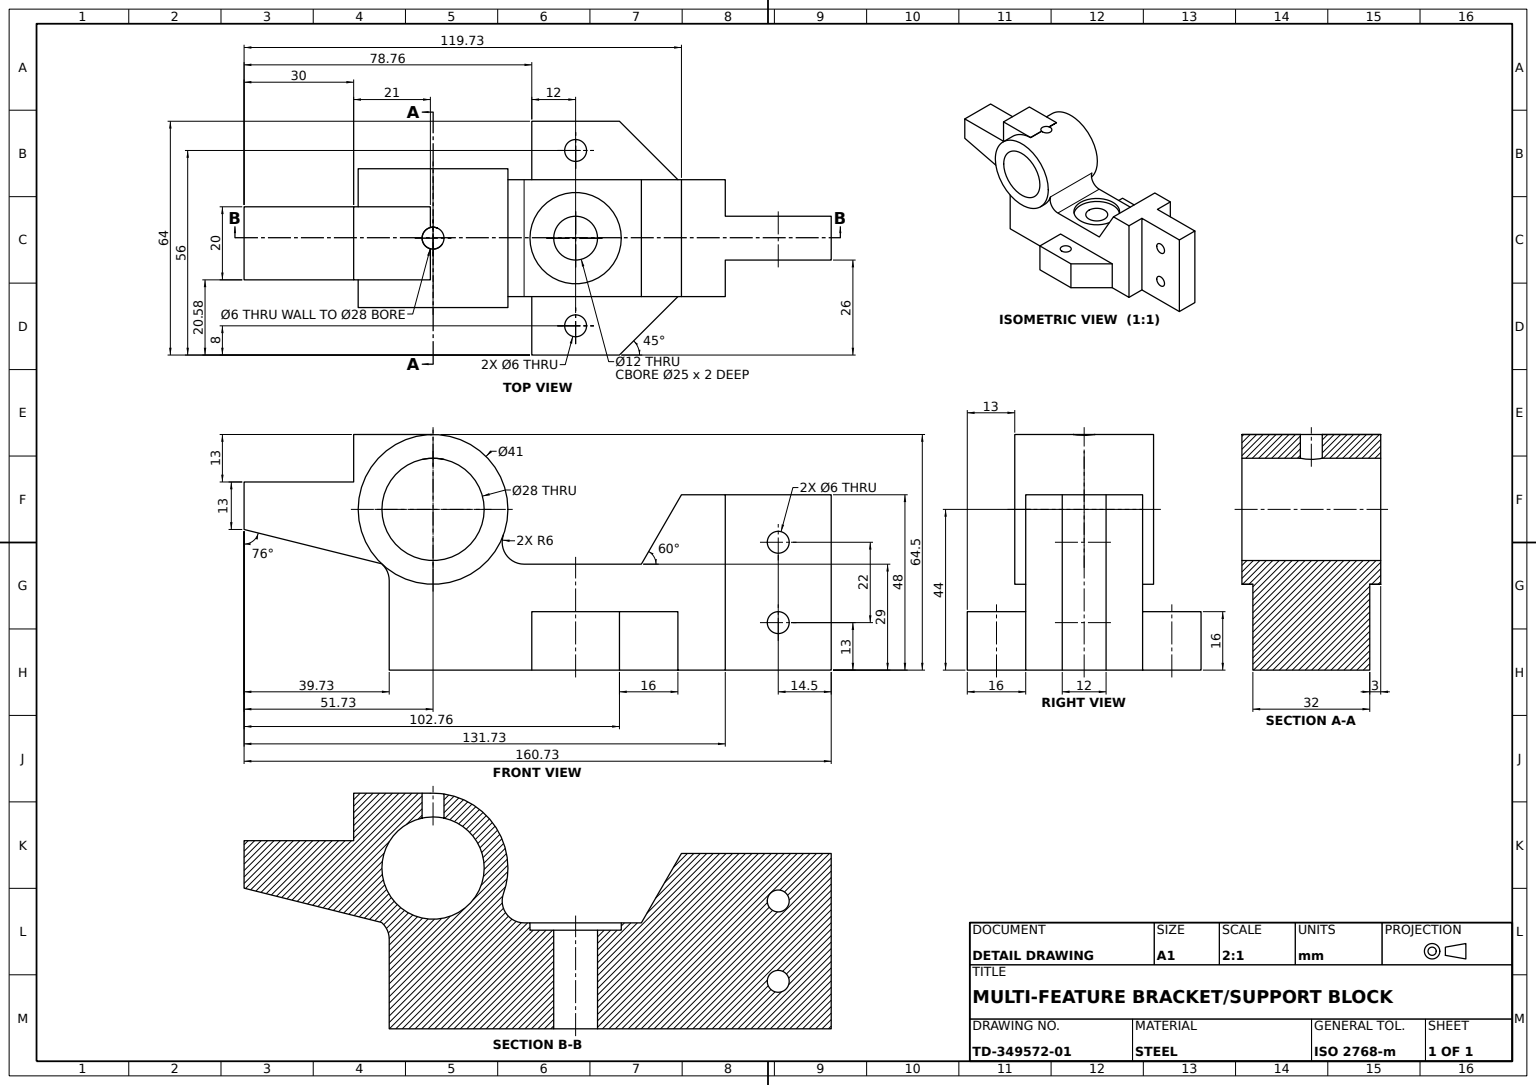
from build123d import *
from build123d.topology import SkipClean

# Parameters (mm, degrees)
PEDESTAL_PROFILE_SKETCH_R       = 14
PEDESTAL_BODY_DEPTH             = 32
VERTICAL_BORE_SKETCH_R          = 6
VERTICAL_BORE_16_DEPTH          = 32
COUNTERBORE_SKETCH_R            = 12.5
COUNTERBORE_25X2_DEPTH          = 2
SIDE_MOUNTING_BLOCK_SKETCH_W    = 29
SIDE_MOUNTING_BLOCK_SKETCH_H    = 12
SIDE_MOUNTING_BLOCK_DEPTH       = 48
BLOCK_MOUNTING_HOLES_SKETCH_R   = 3
BLOCK_MOUNTING_HOLES_2X_6_DEPTH = 48
T_SLOT_FLANGE_SKETCH_R          = 3
T_SLOT_FLANGE_DEPTH             = 16
TOP_HOLE_SKETCH_R               = 3
TOP_HOLE_6_DEPTH                = 16
UPPER_ARM_BLOCK_DEPTH           = 13
TRUNNION_START                  = -60
TRUNNION_BORE_SKETCH_A_R        = 14
TRUNNION_BORE_28_A_DEPTH        = 60
UPPER_ARM_EXTENSION_SKETCH_W    = 30
UPPER_ARM_EXTENSION_SKETCH_H    = 20
UPPER_ARM_EXTENSION_SKETCH_W_2  = 6.345868722
UPPER_ARM_EXTENSION_SKETCH_W_3  = 2.654131278
UPPER_ARM_EXTENSION_DEPTH       = 13
ANGLED_START                    = -20
ANGLED_SIDE_LUG_DEPTH           = 20
TRUNNION_BORE_SKETCH_B_R        = 14
TRUNNION_BORE_28_B_DEPTH        = 60
BORE_COLLAR_SKETCH_A_R          = 20.5
BORE_COLLAR_SKETCH_A_R_2        = 14
BORE_COLLAR_41X3_A_DEPTH        = 3
BORE_START                      = 3
BORE_COLLAR_SKETCH_B_R          = 20.5
BORE_COLLAR_SKETCH_B_R_2        = 14
BORE_COLLAR_41X3_B_DEPTH        = 3


with BuildPart() as part:
    # Pedestal Profile Sketch → Pedestal Body (new body)
    with BuildSketch(Plane.XY):
        with BuildLine():
            Line((-46, 0), (46, 0))
            Line((46, 0), (46, 48))
            Line((46, 48), (34, 48))
            Line((34, 48), (23.030344885, 29))
            Line((23.030344885, 29), (-9.075112839, 29))
            ThreePointArc((-9.075112839, 29), (-13.985632928, 31.552277208), (-14.718483517, 37.037735849))
            ThreePointArc((-14.718483517, 37.037735849), (-38.848476276, 63.918390442), (-47.924528302, 28.954817662))
            ThreePointArc((-47.924528302, 28.954817662), (-46.5021445, 26.954178183), (-46, 24.551349661))
            Line((-46, 24.551349661), (-46, 0))
        make_face()
        with Locations((-34, 44)):
            Circle(PEDESTAL_PROFILE_SKETCH_R, mode=Mode.SUBTRACT)
    extrude(amount=PEDESTAL_BODY_DEPTH)

    # Vertical Bore Sketch → Vertical Bore Ø16 (cut)
    with BuildSketch(Plane(origin=(0, 29, 0), x_dir=(1, 0, 0), z_dir=(0, 1, 0))):
        with Locations(Location((5.030344885, -16, 0), (0, 0, 180))):
            Circle(VERTICAL_BORE_SKETCH_R)
    extrude(amount=-VERTICAL_BORE_16_DEPTH, mode=Mode.SUBTRACT)

    # Counterbore Sketch → Counterbore Ø25x2 (cut)
    with BuildSketch(Plane(origin=(0, 29, 0), x_dir=(1, 0, 0), z_dir=(0, 1, 0))):
        with Locations(Location((5.030344885, -16, 0), (0, 0, 180))):
            Circle(COUNTERBORE_SKETCH_R)
    extrude(amount=-COUNTERBORE_25X2_DEPTH, mode=Mode.SUBTRACT)

    # Side Mounting Block Sketch → Side Mounting Block (add)
    with BuildSketch(Plane(origin=(0, 48, 0), x_dir=(1, 0, 0), z_dir=(0, 1, 0))):
        with Locations((60.5, -16)):
            Rectangle(SIDE_MOUNTING_BLOCK_SKETCH_W, SIDE_MOUNTING_BLOCK_SKETCH_H)
    extrude(amount=-SIDE_MOUNTING_BLOCK_DEPTH)

    # Block Mounting Holes Sketch → Block Mounting Holes 2xØ6 (cut)
    with BuildSketch(Plane.XY.offset(22)):
        with Locations((60.5, 35)):
            Circle(BLOCK_MOUNTING_HOLES_SKETCH_R)
        with Locations((60.5, 13)):
            Circle(BLOCK_MOUNTING_HOLES_SKETCH_R)
    extrude(amount=-BLOCK_MOUNTING_HOLES_2X_6_DEPTH, mode=Mode.SUBTRACT)

    # T-Slot Flange Sketch → T-Slot Flange (add)
    # profile 1 of 2: a face of its own
    with BuildSketch(Plane.XZ):
        Polygon((-6.969655115, -16), (-6.969655115, 0), (33.030344885, 0), (17.030344885, -16), align=None)
        with Locations(Location((5.030344885, -8, 0), (0, 0, 270))):
            Circle(T_SLOT_FLANGE_SKETCH_R, mode=Mode.SUBTRACT)
    # profile 2 of 2: a face of its own
    with BuildSketch(Plane.XZ):
        Polygon((17.030344885, 48), (-6.969655115, 48), (-6.969655115, 32), (33.030344885, 32), align=None)
        with Locations(Location((5.030344885, 40, 0), (0, 0, 270))):
            Circle(T_SLOT_FLANGE_SKETCH_R, mode=Mode.SUBTRACT)
    extrude(amount=-T_SLOT_FLANGE_DEPTH)

    # Top Hole Sketch → Top Hole Ø6 (cut)
    with BuildSketch(Plane(origin=(0, 64.5, 0), x_dir=(1, 0, 0), z_dir=(0, 1, 0))):
        with Locations(Location((-34, -16, 0), (0, 0, 270))):
            Circle(TOP_HOLE_SKETCH_R)
    extrude(amount=-TOP_HOLE_6_DEPTH, mode=Mode.SUBTRACT)

    # Upper Arm Block Sketch → Upper Arm Block (add)
    with BuildSketch(Plane(origin=(0, 64.5, 0), x_dir=(1, 0, 0), z_dir=(0, 1, 0))):
        with BuildLine():
            Line((-34.732915306, -7.416104235), (-55.732915306, -7.416104235))
            Line((-55.732915306, -7.416104235), (-55.732915306, -27.416104235))
            Line((-55.732915306, -27.416104235), (-34.732915306, -27.416104235))
            Line((-34.732915306, -27.416104235), (-34.732915306, -18.909095247))
            ThreePointArc((-34.732915306, -18.909095247), (-37, -16), (-34.732915306, -13.090904753))
            Line((-34.732915306, -13.090904753), (-34.732915306, -7.416104235))
        make_face()
    extrude(amount=-UPPER_ARM_BLOCK_DEPTH)

    # Trunnion Bore Sketch A → Trunnion Bore Ø28 A (cut)
    with BuildSketch(Plane.XY.offset(32).offset(TRUNNION_START)):
        with Locations((-34, 44)):
            Circle(TRUNNION_BORE_SKETCH_A_R)
    extrude(amount=TRUNNION_BORE_28_A_DEPTH, mode=Mode.SUBTRACT)

    # Upper Arm Extension Sketch → Upper Arm Extension (add)
    with BuildSketch(Plane.XZ.offset(-51.5)):
        with Locations((-70.732915306, 17.416104235)):
            Rectangle(UPPER_ARM_EXTENSION_SKETCH_W, UPPER_ARM_EXTENSION_SKETCH_H)
        with Locations((-49.905849667, 17.416104235)):
            Rectangle(UPPER_ARM_EXTENSION_SKETCH_W_2, UPPER_ARM_EXTENSION_SKETCH_H)
        with Locations((-54.405849667, 17.416104235)):
            Rectangle(UPPER_ARM_EXTENSION_SKETCH_W_3, UPPER_ARM_EXTENSION_SKETCH_H)
    extrude(amount=UPPER_ARM_EXTENSION_DEPTH)

    # Angled Side Lug Sketch → Angled Side Lug (add)
    with BuildSketch(Plane.XY.offset(27.416104235).offset(ANGLED_START)):
        with BuildLine():
            Line((-85.732915306, 38.5), (-48.097020916, 29.116317616))
            ThreePointArc((-48.097020916, 29.116317616), (-51.561087718, 33.423696385), (-53.748417658, 38.5))
            Line((-53.748417658, 38.5), (-85.732915306, 38.5))
        make_face()
    extrude(amount=ANGLED_SIDE_LUG_DEPTH)

    # Trunnion Bore Sketch B → Trunnion Bore Ø28 B (cut)
    with BuildSketch(Plane.XY.offset(32).offset(TRUNNION_START)):
        with Locations((-34, 44)):
            Circle(TRUNNION_BORE_SKETCH_B_R)
    extrude(amount=TRUNNION_BORE_28_B_DEPTH, mode=Mode.SUBTRACT)

    # Bore Collar Sketch A → Bore Collar Ø41x3 A (add)
    with BuildSketch(Plane.XY.offset(32)):
        with Locations(Location((-34, 44, 0), (0, 0, 227.215305089))):
            Circle(BORE_COLLAR_SKETCH_A_R)
        with Locations((-34, 44)):
            Circle(BORE_COLLAR_SKETCH_A_R_2, mode=Mode.SUBTRACT)
    extrude(amount=BORE_COLLAR_41X3_A_DEPTH)

    # Bore Collar Sketch B → Bore Collar Ø41x3 B (add)
    with SkipClean():  # the faces are left unmerged after this step: merging them gives an invalid solid
        with BuildSketch(Plane(origin=(0, 0, 0), x_dir=(-1, 0, 0), z_dir=(0, 0, -1)).offset(BORE_START)):
            with Locations((34, 44)):
                Circle(BORE_COLLAR_SKETCH_B_R)
            with Locations((34, 44)):
                Circle(BORE_COLLAR_SKETCH_B_R_2, mode=Mode.SUBTRACT)
        extrude(amount=-BORE_COLLAR_41X3_B_DEPTH)


solid = part.part
